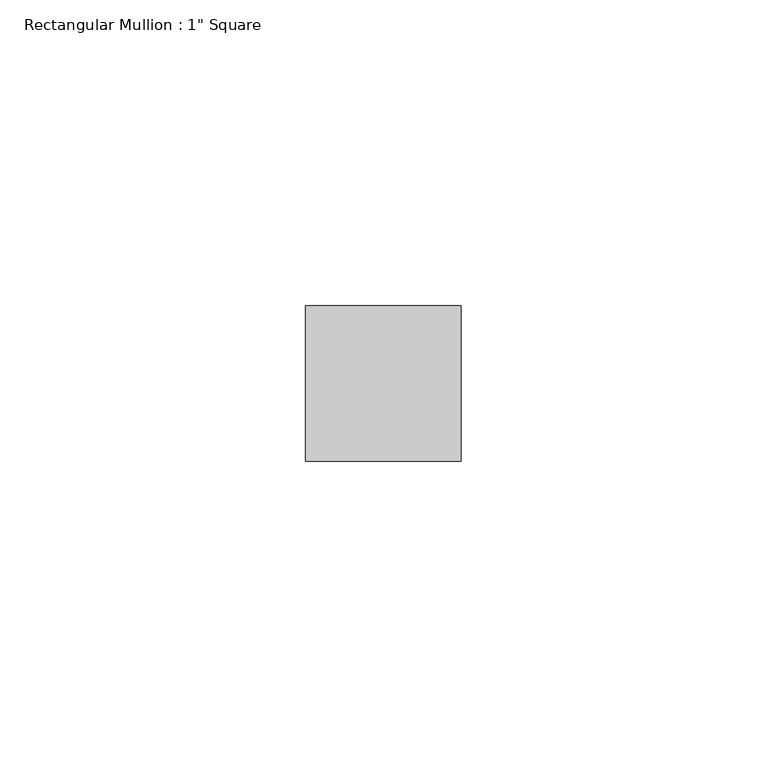
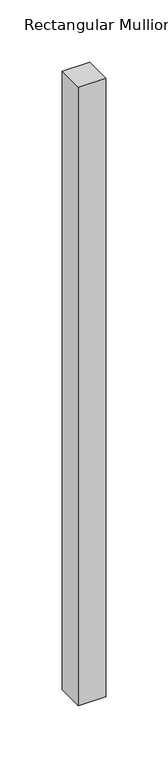
"""IFC4 building model written with IfcOpenShell, lengths in millimetres: member geometry."""

from ifc_helpers import new_model, si_unit, frame, origin, place, context, project, spatial, polyline, outline, extrude, source, transform, mapped, element, save


def member_968ff67a(model_context):
    return source(origin(), model_context, "Body", "SweptSolid", [
        extrude(outline(polyline([(12.7, 12.7), (12.7, -12.7), (-12.7, -12.7), (-12.7, 12.7), (12.7, 12.7)])), frame((0.0, 0.0, -605.3666667), z_axis=(0.0, 0.0, 1.0), x_axis=(1.0, 0.0, 0.0)), (0.0, 0.0, 1.0), 605.3666667),
    ])


if __name__ == "__main__":
    model = new_model("IFC4")
    model_context = context("Model", 3, world=origin())
    ifc_project = project(units=[si_unit("LENGTHUNIT", "METRE", prefix="MILLI")], contexts=[model_context])
    site = spatial("IfcSite", under=ifc_project)
    building = spatial("IfcBuilding", under=site)
    placement = place(None, origin())
    member_shape = member_968ff67a(model_context)
    element("IfcMember", 1, ObjectType="Rectangular Mullion : 1\" Square", at=placement, inside=building, context=model_context, shape_type="MappedRepresentation", body=[
        mapped(member_shape, transform((0.0, 0.0, 0.0), x_axis=(1.0, 0.0, 0.0), y_axis=(0.0, 1.0, 0.0), z_axis=(0.0, 0.0, 1.0))),
    ])
    save(model, "model.ifc")

# Revit data of these elements
# Type "Rectangular Mullion : 1\" Square"
#   built-in parameter 1007304 = 0.0833333 (stored number, unit not read)
#   built-in parameter 1007301 = 0.0416667 (stored number, unit not read)
#   built-in parameter 1007300 = 0.0416667 (stored number, unit not read)
# Element 1 (IfcMember, "Rectangular Mullion : 1\" Square")
#   Materials on its faces: "Aluminum"
# Materials
#   "Aluminum": class "Metal", colour RGB 247 247 247, transparency 0, Description = "Aluminum 6061", Cost = 0
